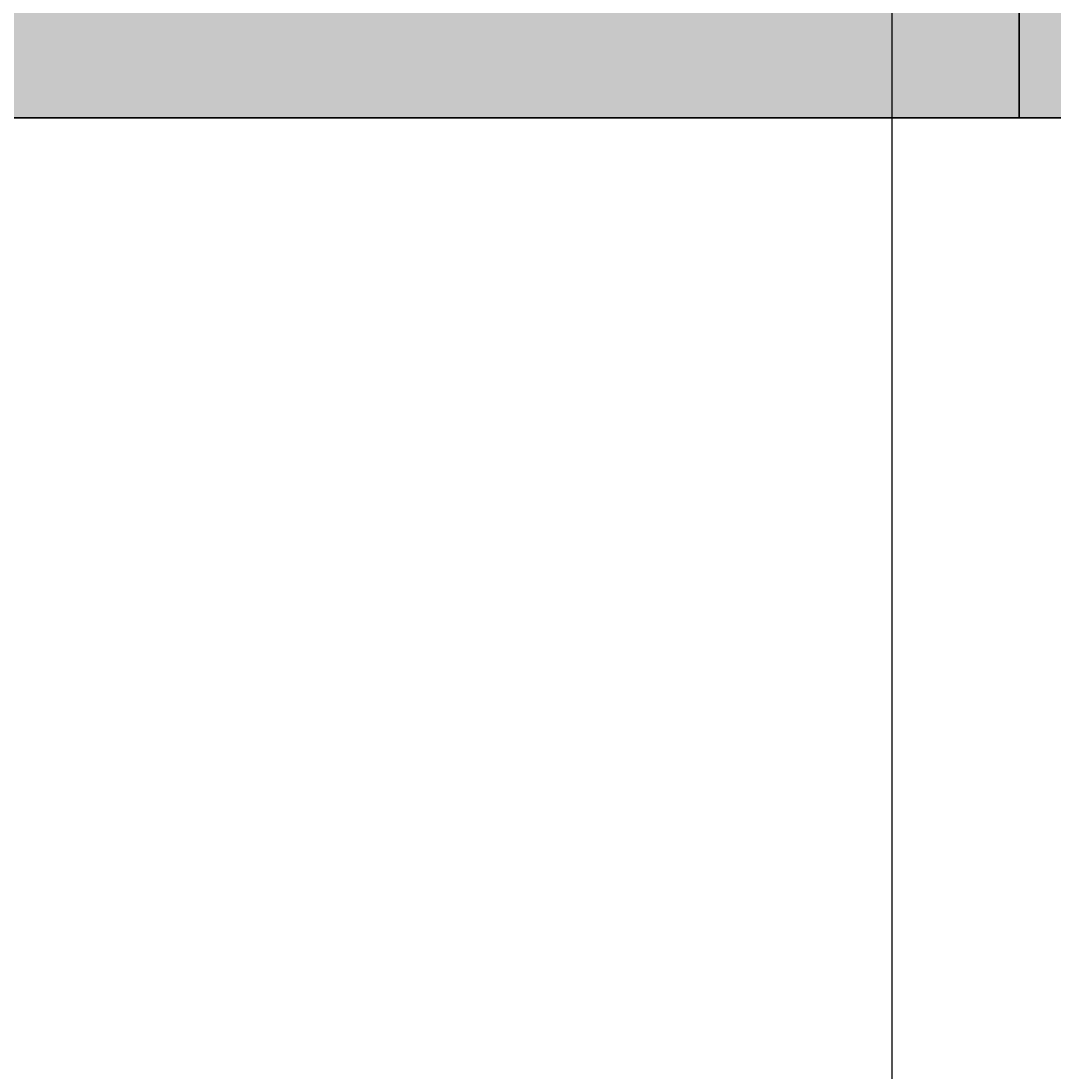
# Model space of a CAD drawing. Units: inches. Extents: x 1998 to 2588, y 1139 to 1977.
# Tile 31 of 134: x 2257 to 2293, y 1484 to 1522. Entities that reach past the tile are written whole.
import ezdxf

# ---------------------------------------------------------------- set-up
doc = ezdxf.new("R2010")
doc.units = ezdxf.units.IN
for name, color, linetype, lineweight in [('A-ANNO-DIMS', 2, 'Continuous', 18), ('A-WALL-PATT', 252, 'Continuous', 13), ('WALL', 200, 'Continuous', 35)]:
    doc.layers.add(name, color=color, linetype=linetype, lineweight=lineweight)
doc.styles.get("Standard").update_dxf_attribs({"font": 'arial.ttf'})
doc.dimstyles.get("Standard").update_dxf_attribs({"dimtxt": 0.18, "dimasz": 0.18, "dimexe": 0.18, "dimexo": 0.0625, "dimgap": 0.09, "dimtad": 0, "dimtih": 1, "dimtoh": 1, "dimdec": 4, "dimzin": 0, "dimdsep": 46, "dimtxsty": 'Standard', "dimcen": 0.09, "dimadec": 0, "dimazin": 0, "dimtfac": 1, "dimtdec": 4, "dimtofl": 0, "dimtmove": 0, "dimatfit": 3, "dimfxl": 1, "dimtolj": 1, "dimtzin": 0, "dimarcsym": 0})

# ---------------------------------------------------------------- blocks, each defined once
blk = doc.blocks.new('*D41')
at = {"layer": 'A-ANNO-DIMS', "color": 0, "lineweight": -2, "transparency": 16777216}
for p, q in [((2227.473, 1588.67), (2227.473, 1138.602)), ((2287.473, 1588.67), (2287.473, 1138.602)), ((2227.653, 1138.782), (2257.254, 1138.782)), ((2287.293, 1138.782), (2257.692, 1138.782))]:
    blk.add_line(p, q, dxfattribs=at)
at = {"layer": 'A-ANNO-DIMS', "color": 0, "transparency": 16777216}
for points in [[(2227.653, 1138.812), (2227.653, 1138.752), (2227.473, 1138.782)], [(2287.293, 1138.812), (2287.293, 1138.752), (2287.473, 1138.782)]]:
    blk.add_solid(points, dxfattribs=at)
at = {"layer": 'Defpoints', "color": 0, "transparency": 16777216}
for p in [(2227.473, 1588.732), (2287.473, 1588.732), (2287.473, 1138.782)]:
    blk.add_point(p, dxfattribs=at)
at = {"layer": 'A-ANNO-DIMS', "color": 0, "transparency": 16777216, "insert": (2257.473, 1138.782), "char_height": 0.18, "attachment_point": 5}
blk.add_mtext('\\A1;60', dxfattribs=at)

msp = doc.modelspace()

# ---------------------------------------------------------------- hatches: boundary and pattern name
at = {"layer": 'A-WALL-PATT'}
h = msp.add_hatch(color=256, dxfattribs=at)
h.dxf.hatch_style = 1
h.paths.add_polyline_path([(2222.9729, 1888.7324), (2099.4125, 1888.7324), (2099.4125, 1879.7324), (2222.9729, 1879.7324)])
h.paths.add_polyline_path([(2096.9729, 1868.3278), (2087.9729, 1868.3278), (2087.9729, 1775.637), (2096.9729, 1775.637)])
h.paths.add_polyline_path([(2227.4729, 1868.3278), (2222.9729, 1868.3278), (2222.9729, 1774.3318), (2227.4729, 1774.3318)])
h.paths.add_polyline_path([(2188.3019, 1759.7324), (2138.6074, 1759.7324), (2099.4125, 1759.7324), (2099.4125, 1755.2324), (2176.9729, 1755.2324), (2188.3019, 1755.2324)])
h.paths.add_polyline_path([(2087.9729, 1759.7324), (2059.4729, 1759.7324), (2059.4729, 1702.7324), (2087.9729, 1702.7324), (2087.9729, 1707.2324), (2063.9729, 1707.2324), (2063.9729, 1755.2324), (2087.9729, 1755.2324)])
h.paths.add_polyline_path([(2096.9729, 1755.2324), (2087.9729, 1755.2324), (2087.9729, 1707.2324), (2096.9729, 1707.2324)])
h.paths.add_polyline_path([(2187.0461, 1707.2324), (2105.9729, 1707.2324), (2096.9729, 1707.2324), (2087.9729, 1707.2324), (2087.9729, 1702.7324), (2105.9729, 1702.7324), (2114.9729, 1702.7324), (2187.0461, 1702.7324)])
h.paths.add_polyline_path([(2181.4729, 1719.2028), (2176.9729, 1719.2028), (2176.9729, 1707.2324), (2181.4729, 1707.2324)])
h.paths.add_polyline_path([(2216.0332, 1588.7324), (2114.9729, 1588.7324), (2105.9729, 1588.7324), (2105.9729, 1584.2324), (2216.0332, 1584.2324)])
h.paths.add_polyline_path([(2077.691, 1588.7324), (2061.4729, 1588.7324), (2061.4729, 1584.2324), (2077.691, 1584.2324)])
h.paths.add_polyline_path([(2105.9729, 1588.7324), (2098.0956, 1588.7324), (2098.0956, 1584.2324), (2105.9729, 1584.2324)])
h.paths.add_polyline_path([(2114.9729, 1596.2642), (2110.1012, 1596.2642), (2105.9729, 1596.2642), (2105.9729, 1588.7324), (2114.9729, 1588.7324)])
h.paths.add_polyline_path([(2114.9729, 1584.2324), (2105.9729, 1584.2324), (2105.9729, 1580.249), (2110.1012, 1580.249), (2114.9729, 1580.249)])
h.paths.add_polyline_path([(2114.9729, 1547.7716), (2110.1012, 1547.7716, -0.0318759), (2105.9729, 1548.035), (2105.9729, 1470.2324), (2108.3775, 1470.2324), (2108.3775, 1465.7324), (2186.2943, 1465.7324), (2186.2943, 1470.2324), (2114.9729, 1470.2324)])
h.paths.add_polyline_path([(2227.4729, 1584.2324), (2222.9729, 1584.2324), (2222.9729, 1486.137), (2227.4729, 1486.137)])
h.paths.add_polyline_path([(2295.4138, 1593.2324), (2227.4729, 1593.2324), (2227.4729, 1588.7324), (2295.4138, 1588.7324), (2295.4138, 1591.8729)])
h.paths.add_polyline_path([(2345.9729, 1627.1165), (2341.4729, 1627.1165), (2341.4729, 1593.2324), (2337.2869, 1593.2324), (2337.2869, 1591.8729), (2337.2869, 1588.7324), (2345.9729, 1588.7324)])
h.paths.add_polyline_path([(2291.9729, 1588.7324), (2287.4729, 1588.7324), (2287.4729, 1522.7324), (2291.9729, 1522.7324)])
h.paths.add_polyline_path([(2291.9729, 1522.7324), (2287.4729, 1522.7324), (2227.4729, 1522.7324), (2227.4729, 1518.2324), (2291.9729, 1518.2324)])
h.paths.add_polyline_path([(2295.7347, 1519.5919), (2295.7347, 1522.7324), (2291.9729, 1522.7324), (2291.9729, 1518.2324), (2295.7347, 1518.2324)])
h.paths.add_polyline_path([(2345.9729, 1522.7324), (2337.6078, 1522.7324), (2337.6078, 1519.5919), (2337.6078, 1518.2324), (2341.4729, 1518.2324), (2341.4729, 1488.5616), (2345.9729, 1488.5616)])
h.paths.add_polyline_path([(2345.9729, 1468.1569), (2341.4729, 1468.1569), (2341.4729, 1374.2324), (2227.4729, 1374.2324), (2227.4729, 1369.7324), (2345.9729, 1369.7324)])
h.paths.add_polyline_path([(2345.9729, 1369.7324), (2341.4729, 1369.7324), (2341.4729, 1362.2324), (2345.9729, 1362.2324)])
h.paths.add_polyline_path([(2345.9729, 1317.7324), (2345.9729, 1322.2324), (2341.4729, 1322.2324), (2341.4729, 1285.137), (2345.9729, 1285.137)], flags=17)
h.paths.add_polyline_path([(2356.2096, 1322.2324), (2345.9729, 1322.2324), (2345.9729, 1317.7324), (2356.2096, 1317.7324), (2356.2096, 1319.3088)], flags=17)
h.paths.add_polyline_path([(2393.9729, 1322.2324), (2375.6999, 1322.2324), (2375.6999, 1319.3088, -0.0202458), (2375.636, 1317.7324), (2393.9729, 1317.7324)], flags=17)
h.paths.add_polyline_path([(2398.4729, 1322.2324), (2393.9729, 1322.2324), (2393.9729, 1317.7324), (2393.9729, 1237.7324), (2345.9729, 1237.7324), (2345.9729, 1264.7324), (2341.4729, 1264.7324), (2341.4729, 1228.7324), (2393.9729, 1228.7324), (2482.7412, 1228.7324), (2482.7412, 1237.7324), (2398.4729, 1237.7324), (2398.4729, 1297.1029)])
h.paths.add_polyline_path([(2398.4729, 1362.2324), (2393.9729, 1362.2324), (2393.9729, 1357.7324), (2398.4729, 1357.7324)])
h.paths.add_polyline_path([(2345.9729, 1329.7549), (2341.4729, 1329.7549), (2341.4729, 1322.2324), (2345.9729, 1322.2324)])

# ---------------------------------------------------------------- linework, layer by layer
at = {"layer": 'WALL'}
for p, q in [((2291.9729, 1518.2324), (2291.9729, 1588.7324)), ((2227.4729, 1518.2324), (2291.9729, 1518.2324)), ((2227.4729, 1518.2324), (2296.6507, 1518.2324))]:
    msp.add_line(p, q, dxfattribs=at)

# ---------------------------------------------------------------- dimensions: what is measured, and where the dimension line sits
at = {"layer": 'A-ANNO-DIMS'}
dim = msp.add_linear_dim(base=(2287.4729, 1138.7824), p1=(2227.4729, 1588.7324), p2=(2287.4729, 1588.7324), dimstyle='Standard', override={"dimdec": 0, "dimlfac": 1, "dimrnd": 0, "dimzin": 0, "dimdsep": 46, "dimlunit": 2}, dxfattribs=at)
dim.commit()
dim.dimension.update_dxf_attribs({"geometry": '*D41', "text_midpoint": (2257.4729, 1138.7824)})

doc.saveas('drawing.dxf')
